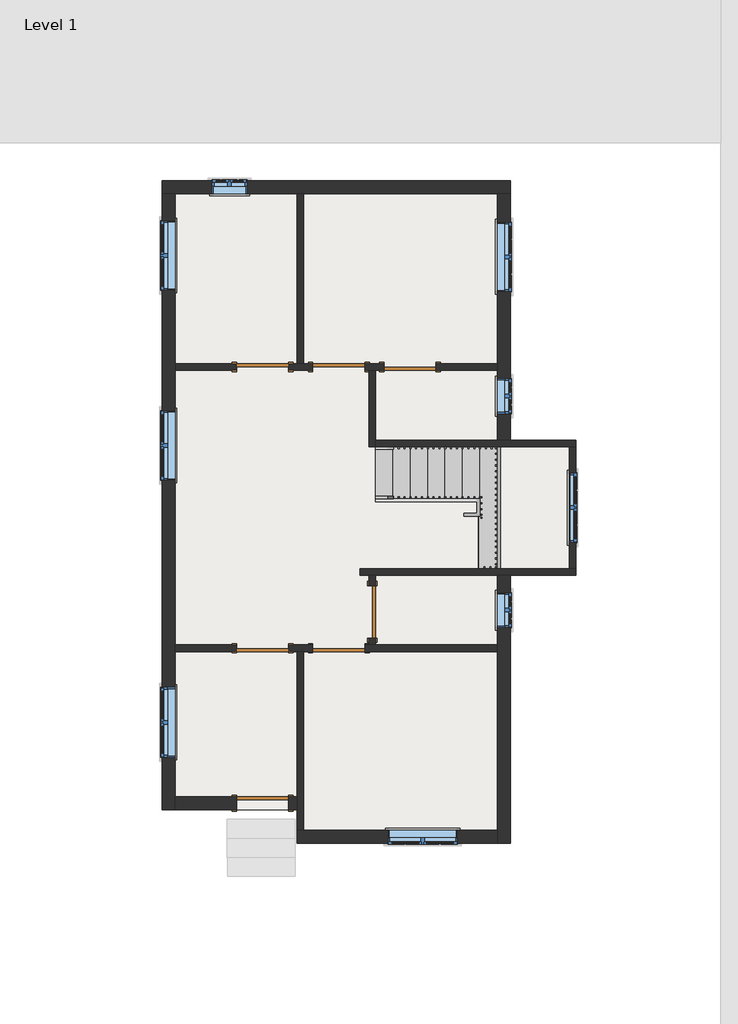
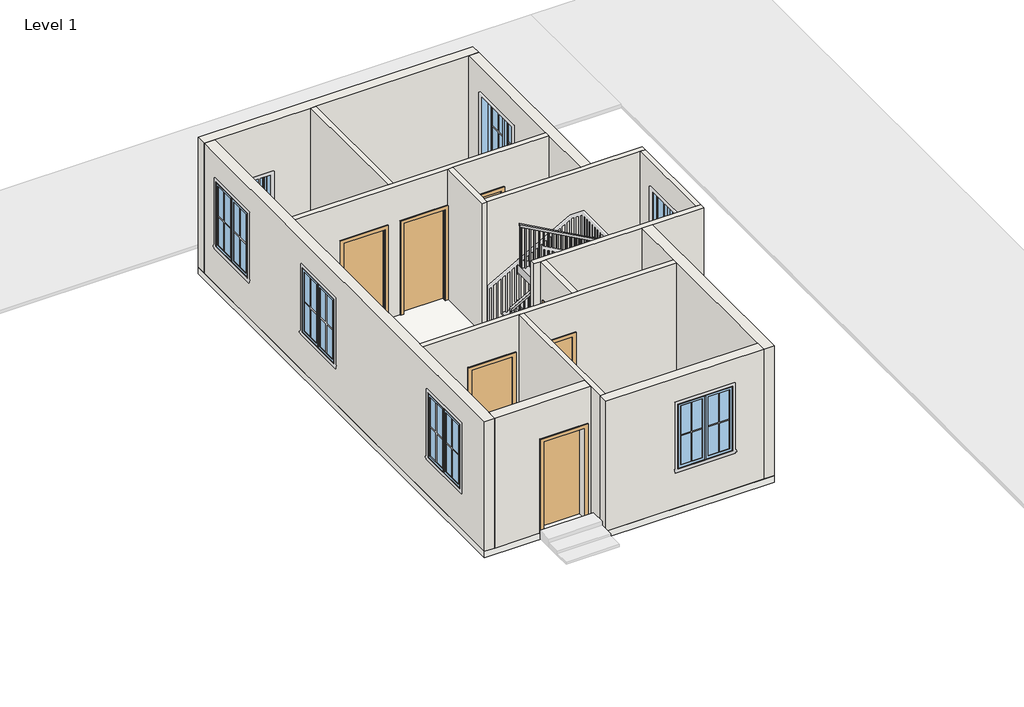
# One storey, part 1 of 2: 15 walls, 9 windows, 7 doors, 1 railing, 1 slab, 1 stair flight.
"""IFC4 building model written with IfcOpenShell, lengths in millimetres."""

from ifc_helpers import new_model, si_unit, frame, origin, origin_with_axes, place, context, project, spatial, polyline, outline, extrude, faceted_brep, transform, mapped, element, save
from components import door_e5f9f3c4, door_305aa2a5, door_0ca8825f, stair_flight_65dd4c8f, window_c417fced, window_8377141f, window_d9d3dda5

model = new_model("IFC4")

# Units and contexts
model_context = context("Model", 3, world=origin())
ifc_project = project(units=[si_unit("LENGTHUNIT", "METRE", prefix="MILLI")], contexts=[model_context])

# Site, building, storey
site = spatial("IfcSite", under=ifc_project)
building = spatial("IfcBuilding", under=site)
storey = spatial("IfcBuildingStorey", under=building, Name="Level 1", Elevation=0.0)

# Doors
placement = place(None, origin())
door_shape = door_e5f9f3c4(model_context)
element("IfcDoor", 1, ObjectType="Single-Flush : 36\" x 84\"", at=placement, inside=storey, context=model_context, shape_type="MappedRepresentation", body=[
    mapped(door_shape, transform((3028.95, 10966.45, 0.0), x_axis=(1.0, 0.0, 0.0), y_axis=(0.0, 1.0, 0.0), z_axis=(0.0, 0.0, 1.0))),
])
element("IfcDoor", 2, ObjectType="Single-Flush : 36\" x 84\"", at=placement, inside=storey, context=model_context, shape_type="MappedRepresentation", body=[
    mapped(door_shape, transform((5607.05, 10966.45, 0.0), x_axis=(-1.0, 0.0, 0.0), y_axis=(0.0, -1.0, 0.0), z_axis=(0.0, 0.0, 1.0))),
])
element("IfcDoor", 3, ObjectType="Single-Flush : 36\" x 84\"", at=placement, inside=storey, context=model_context, shape_type="MappedRepresentation", body=[
    mapped(door_shape, transform((4362.45, 6051.55, 0.0), x_axis=(-1.0, 0.0, 0.0), y_axis=(0.0, -1.0, 0.0), z_axis=(0.0, 0.0, 1.0))),
])
element("IfcDoor", 4, ObjectType="Single-Flush : 36\" x 84\"", at=placement, inside=storey, context=model_context, shape_type="MappedRepresentation", body=[
    mapped(door_shape, transform((4946.65, 6686.55, 0.0), x_axis=(0.0, -1.0, 0.0), y_axis=(1.0, 0.0, 0.0), z_axis=(0.0, 0.0, 1.0))),
])
door_2_shape = door_305aa2a5(model_context)
element("IfcDoor", 5, ObjectType="Single-Flush : 36\" x 84\"", at=placement, inside=storey, context=model_context, shape_type="MappedRepresentation", body=[
    mapped(door_2_shape, transform((4362.45, 10966.45, 0.0), x_axis=(-1.0, 0.0, 0.0), y_axis=(0.0, -1.0, 0.0), z_axis=(0.0, 0.0, 1.0))),
])
element("IfcDoor", 6, ObjectType="Single-Flush : 36\" x 84\"", at=placement, inside=storey, context=model_context, shape_type="MappedRepresentation", body=[
    mapped(door_2_shape, transform((3028.95, 6051.55, 0.0), x_axis=(1.0, 0.0, 0.0), y_axis=(0.0, 1.0, 0.0), z_axis=(0.0, 0.0, 1.0))),
])
door_3_shape = door_0ca8825f(model_context)
element("IfcDoor", 7, ObjectType="Single-Flush : 36\" x 84\"", at=placement, inside=storey, context=model_context, shape_type="MappedRepresentation", body=[
    mapped(door_3_shape, transform((3028.95, 3340.1, 0.0), x_axis=(1.0, 0.0, 0.0), y_axis=(0.0, 1.0, 0.0), z_axis=(0.0, 0.0, 1.0))),
])

# Railing
element("IfcRailing", 8, ObjectType="Handrail - Rectangular", at=placement, inside=storey, context=model_context, shape_type="SolidModel", body=[
    faceted_brep([(5003.8, 8712.2, 1083.7333333), (5003.8, 8712.2, 1025.620221), (5003.8, 8661.4, 1025.620221), (5003.8, 8661.4, 1083.7333333), (6756.4, 8712.2, 2057.4), (6807.2, 8712.2, 2027.5091099), (6807.2, 8661.4, 2027.5091099), (6756.4, 8661.4, 2057.4), (6756.4, 8712.2, 2099.7333333), (6807.2, 8712.2, 2048.9333333), (6807.2, 8661.4, 2048.9333333), (6756.4, 8661.4, 2099.7333333), (6883.4, 8712.2, 2099.7333333), (6883.4, 8712.2, 2048.9333333), (6832.6, 8661.4, 2048.9333333), (6832.6, 8661.4, 2099.7333333), (6883.4, 8585.2, 2099.7333333), (6883.4, 8585.2, 2048.9333333), (6832.6, 8585.2, 2048.9333333), (6832.6, 8585.2, 2099.7333333), (6883.4, 8432.8, 2099.7333333), (6883.4, 8382.0, 2048.9333333), (6832.6, 8382.0, 2048.9333333), (6832.6, 8432.8, 2099.7333333), (6883.4, 8432.8, 2311.4), (6883.4, 8382.0, 2260.6), (6832.6, 8382.0, 2260.6), (6832.6, 8432.8, 2311.4), (6883.4, 8305.8, 2311.4), (6883.4, 8305.8, 2260.6), (6832.6, 8356.6, 2260.6), (6832.6, 8356.6, 2311.4), (6756.4, 8305.8, 2311.4), (6743.2363978, 8305.8, 2260.6), (6743.2363978, 8356.6, 2260.6), (6756.4, 8356.6, 2311.4), (5003.8, 8305.8, 3285.0666667), (5003.8, 8356.6, 3285.0666667), (5003.8, 8356.6, 3226.9535543), (5003.8, 8305.8, 3226.9535543)], [[[0, 1, 2, 3]], [[1, 0, 4, 5]], [[2, 1, 5, 6]], [[3, 2, 6, 7]], [[0, 3, 7, 4]], [[5, 4, 8, 9]], [[6, 5, 9, 10]], [[7, 6, 10, 11]], [[4, 7, 11, 8]], [[9, 8, 12, 13]], [[10, 9, 13, 14]], [[11, 10, 14, 15]], [[8, 11, 15, 12]], [[13, 12, 16, 17]], [[14, 13, 17, 18]], [[15, 14, 18, 19]], [[12, 15, 19, 16]], [[17, 16, 20, 21]], [[18, 17, 21, 22]], [[19, 18, 22, 23]], [[16, 19, 23, 20]], [[21, 20, 24, 25]], [[22, 21, 25, 26]], [[23, 22, 26, 27]], [[20, 23, 27, 24]], [[25, 24, 28, 29]], [[26, 25, 29, 30]], [[27, 26, 30, 31]], [[24, 27, 31, 28]], [[29, 28, 32, 33]], [[30, 29, 33, 34]], [[31, 30, 34, 35]], [[28, 31, 35, 32]], [[36, 37, 38, 39]], [[33, 32, 36, 39]], [[34, 33, 39, 38]], [[35, 34, 38, 37]], [[32, 35, 37, 36]]]),
    extrude(outline(polyline([(3207.5507765, 5038.725), (3218.1341099, 5019.675), (2201.3333333, 5019.675), (2201.3333333, 5038.725), (3207.5507765, 5038.725)])), frame((0.0, 8321.675, 0.0), z_axis=(0.0, 1.0, 0.0), x_axis=(0.0, 0.0, 1.0)), (0.0, 0.0, 1.0), 19.05),
    extrude(outline(polyline([(3151.1063321, 5140.325), (3161.6896654, 5121.275), (2201.3333333, 5121.275), (2201.3333333, 5140.325), (3151.1063321, 5140.325)])), frame((0.0, 8321.675, 0.0), z_axis=(0.0, 1.0, 0.0), x_axis=(0.0, 0.0, 1.0)), (0.0, 0.0, 1.0), 19.05),
    extrude(outline(polyline([(3094.6618876, 5241.925), (3105.245221, 5222.875), (2201.3333333, 5222.875), (2201.3333333, 5241.925), (3094.6618876, 5241.925)])), frame((0.0, 8321.675, 0.0), z_axis=(0.0, 1.0, 0.0), x_axis=(0.0, 0.0, 1.0)), (0.0, 0.0, 1.0), 19.05),
    extrude(outline(polyline([(3038.2174432, 5343.525), (3048.8007765, 5324.475), (2032.0, 5324.475), (2032.0, 5343.525), (3038.2174432, 5343.525)])), frame((0.0, 8321.675, 0.0), z_axis=(0.0, 1.0, 0.0), x_axis=(0.0, 0.0, 1.0)), (0.0, 0.0, 1.0), 19.05),
    extrude(outline(polyline([(2981.7729988, 5445.125), (2992.3563321, 5426.075), (2032.0, 5426.075), (2032.0, 5445.125), (2981.7729988, 5445.125)])), frame((0.0, 8321.675, 0.0), z_axis=(0.0, 1.0, 0.0), x_axis=(0.0, 0.0, 1.0)), (0.0, 0.0, 1.0), 19.05),
    extrude(outline(polyline([(2925.3285543, 5546.725), (2935.9118876, 5527.675), (2032.0, 5527.675), (2032.0, 5546.725), (2925.3285543, 5546.725)])), frame((0.0, 8321.675, 0.0), z_axis=(0.0, 1.0, 0.0), x_axis=(0.0, 0.0, 1.0)), (0.0, 0.0, 1.0), 19.05),
    extrude(outline(polyline([(2868.8841099, 5648.325), (2879.4674432, 5629.275), (1862.6666667, 5629.275), (1862.6666667, 5648.325), (2868.8841099, 5648.325)])), frame((0.0, 8321.675, 0.0), z_axis=(0.0, 1.0, 0.0), x_axis=(0.0, 0.0, 1.0)), (0.0, 0.0, 1.0), 19.05),
    extrude(outline(polyline([(2812.4396654, 5749.925), (2823.0229988, 5730.875), (1862.6666667, 5730.875), (1862.6666667, 5749.925), (2812.4396654, 5749.925)])), frame((0.0, 8321.675, 0.0), z_axis=(0.0, 1.0, 0.0), x_axis=(0.0, 0.0, 1.0)), (0.0, 0.0, 1.0), 19.05),
    extrude(outline(polyline([(2755.995221, 5851.525), (2766.5785543, 5832.475), (1862.6666667, 5832.475), (1862.6666667, 5851.525), (2755.995221, 5851.525)])), frame((0.0, 8321.675, 0.0), z_axis=(0.0, 1.0, 0.0), x_axis=(0.0, 0.0, 1.0)), (0.0, 0.0, 1.0), 19.05),
    extrude(outline(polyline([(2699.5507765, 5953.125), (2710.1341099, 5934.075), (1693.3333333, 5934.075), (1693.3333333, 5953.125), (2699.5507765, 5953.125)])), frame((0.0, 8321.675, 0.0), z_axis=(0.0, 1.0, 0.0), x_axis=(0.0, 0.0, 1.0)), (0.0, 0.0, 1.0), 19.05),
    extrude(outline(polyline([(2643.1063321, 6054.725), (2653.6896654, 6035.675), (1693.3333333, 6035.675), (1693.3333333, 6054.725), (2643.1063321, 6054.725)])), frame((0.0, 8321.675, 0.0), z_axis=(0.0, 1.0, 0.0), x_axis=(0.0, 0.0, 1.0)), (0.0, 0.0, 1.0), 19.05),
    extrude(outline(polyline([(2586.6618876, 6156.325), (2597.245221, 6137.275), (1693.3333333, 6137.275), (1693.3333333, 6156.325), (2586.6618876, 6156.325)])), frame((0.0, 8321.675, 0.0), z_axis=(0.0, 1.0, 0.0), x_axis=(0.0, 0.0, 1.0)), (0.0, 0.0, 1.0), 19.05),
    extrude(outline(polyline([(2530.2174432, 6257.925), (2540.8007765, 6238.875), (1524.0, 6238.875), (1524.0, 6257.925), (2530.2174432, 6257.925)])), frame((0.0, 8321.675, 0.0), z_axis=(0.0, 1.0, 0.0), x_axis=(0.0, 0.0, 1.0)), (0.0, 0.0, 1.0), 19.05),
    extrude(outline(polyline([(2473.7729988, 6359.525), (2484.3563321, 6340.475), (1524.0, 6340.475), (1524.0, 6359.525), (2473.7729988, 6359.525)])), frame((0.0, 8321.675, 0.0), z_axis=(0.0, 1.0, 0.0), x_axis=(0.0, 0.0, 1.0)), (0.0, 0.0, 1.0), 19.05),
    extrude(outline(polyline([(2417.3285543, 6461.125), (2427.9118876, 6442.075), (1524.0, 6442.075), (1524.0, 6461.125), (2417.3285543, 6461.125)])), frame((0.0, 8321.675, 0.0), z_axis=(0.0, 1.0, 0.0), x_axis=(0.0, 0.0, 1.0)), (0.0, 0.0, 1.0), 19.05),
    extrude(outline(polyline([(2360.8841099, 6562.725), (2371.4674432, 6543.675), (1354.6666667, 6543.675), (1354.6666667, 6562.725), (2360.8841099, 6562.725)])), frame((0.0, 8321.675, 0.0), z_axis=(0.0, 1.0, 0.0), x_axis=(0.0, 0.0, 1.0)), (0.0, 0.0, 1.0), 19.05),
    extrude(outline(polyline([(2304.4396654, 6664.325), (2315.0229988, 6645.275), (1354.6666667, 6645.275), (1354.6666667, 6664.325), (2304.4396654, 6664.325)])), frame((0.0, 8321.675, 0.0), z_axis=(0.0, 1.0, 0.0), x_axis=(0.0, 0.0, 1.0)), (0.0, 0.0, 1.0), 19.05),
    extrude(outline(polyline([(2247.995221, 6765.925), (2258.5785543, 6746.875), (1354.6666667, 6746.875), (1354.6666667, 6765.925), (2247.995221, 6765.925)])), frame((0.0, 8321.675, 0.0), z_axis=(0.0, 1.0, 0.0), x_axis=(0.0, 0.0, 1.0)), (0.0, 0.0, 1.0), 19.05),
    extrude(outline(polyline([(6848.475, 8391.525), (6867.525, 8391.525), (6867.525, 8372.475), (6848.475, 8372.475), (6848.475, 8391.525)])), frame((0.0, 0.0, 1185.3333333), z_axis=(0.0, 0.0, 1.0), x_axis=(1.0, 0.0, 0.0)), (0.0, 0.0, 1.0), 1075.2666667),
    extrude(outline(polyline([(6848.475, 8493.125), (6867.525, 8493.125), (6867.525, 8474.075), (6848.475, 8474.075), (6848.475, 8493.125)])), frame((0.0, 0.0, 1185.3333333), z_axis=(0.0, 0.0, 1.0), x_axis=(1.0, 0.0, 0.0)), (0.0, 0.0, 1.0), 863.6),
    extrude(outline(polyline([(6848.475, 8594.725), (6867.525, 8594.725), (6867.525, 8575.675), (6848.475, 8575.675), (6848.475, 8594.725)])), frame((0.0, 0.0, 1185.3333333), z_axis=(0.0, 0.0, 1.0), x_axis=(1.0, 0.0, 0.0)), (0.0, 0.0, 1.0), 863.6),
    extrude(outline(polyline([(6823.075, 8677.275), (6823.075, 8696.325), (6842.125, 8696.325), (6842.125, 8677.275), (6823.075, 8677.275)])), frame((0.0, 0.0, 1185.3333333), z_axis=(0.0, 0.0, 1.0), x_axis=(1.0, 0.0, 0.0)), (0.0, 0.0, 1.0), 863.6),
    extrude(outline(polyline([(1990.4674432, 6740.525), (1979.8841099, 6721.475), (1016.0, 6721.475), (1016.0, 6740.525), (1990.4674432, 6740.525)])), frame((0.0, 8677.275, 0.0), z_axis=(0.0, 1.0, 0.0), x_axis=(0.0, 0.0, 1.0)), (0.0, 0.0, 1.0), 19.05),
    extrude(outline(polyline([(1934.0229988, 6638.925), (1923.4396654, 6619.875), (1016.0, 6619.875), (1016.0, 6638.925), (1934.0229988, 6638.925)])), frame((0.0, 8677.275, 0.0), z_axis=(0.0, 1.0, 0.0), x_axis=(0.0, 0.0, 1.0)), (0.0, 0.0, 1.0), 19.05),
    extrude(outline(polyline([(1877.5785543, 6537.325), (1866.995221, 6518.275), (1016.0, 6518.275), (1016.0, 6537.325), (1877.5785543, 6537.325)])), frame((0.0, 8677.275, 0.0), z_axis=(0.0, 1.0, 0.0), x_axis=(0.0, 0.0, 1.0)), (0.0, 0.0, 1.0), 19.05),
    extrude(outline(polyline([(1821.1341099, 6435.725), (1810.5507765, 6416.675), (846.6666667, 6416.675), (846.6666667, 6435.725), (1821.1341099, 6435.725)])), frame((0.0, 8677.275, 0.0), z_axis=(0.0, 1.0, 0.0), x_axis=(0.0, 0.0, 1.0)), (0.0, 0.0, 1.0), 19.05),
    extrude(outline(polyline([(1764.6896654, 6334.125), (1754.1063321, 6315.075), (846.6666667, 6315.075), (846.6666667, 6334.125), (1764.6896654, 6334.125)])), frame((0.0, 8677.275, 0.0), z_axis=(0.0, 1.0, 0.0), x_axis=(0.0, 0.0, 1.0)), (0.0, 0.0, 1.0), 19.05),
    extrude(outline(polyline([(1708.245221, 6232.525), (1697.6618876, 6213.475), (846.6666667, 6213.475), (846.6666667, 6232.525), (1708.245221, 6232.525)])), frame((0.0, 8677.275, 0.0), z_axis=(0.0, 1.0, 0.0), x_axis=(0.0, 0.0, 1.0)), (0.0, 0.0, 1.0), 19.05),
    extrude(outline(polyline([(1651.8007765, 6130.925), (1641.2174432, 6111.875), (677.3333333, 6111.875), (677.3333333, 6130.925), (1651.8007765, 6130.925)])), frame((0.0, 8677.275, 0.0), z_axis=(0.0, 1.0, 0.0), x_axis=(0.0, 0.0, 1.0)), (0.0, 0.0, 1.0), 19.05),
    extrude(outline(polyline([(1595.3563321, 6029.325), (1584.7729988, 6010.275), (677.3333333, 6010.275), (677.3333333, 6029.325), (1595.3563321, 6029.325)])), frame((0.0, 8677.275, 0.0), z_axis=(0.0, 1.0, 0.0), x_axis=(0.0, 0.0, 1.0)), (0.0, 0.0, 1.0), 19.05),
    extrude(outline(polyline([(1538.9118876, 5927.725), (1528.3285543, 5908.675), (677.3333333, 5908.675), (677.3333333, 5927.725), (1538.9118876, 5927.725)])), frame((0.0, 8677.275, 0.0), z_axis=(0.0, 1.0, 0.0), x_axis=(0.0, 0.0, 1.0)), (0.0, 0.0, 1.0), 19.05),
    extrude(outline(polyline([(1482.4674432, 5826.125), (1471.8841099, 5807.075), (508.0, 5807.075), (508.0, 5826.125), (1482.4674432, 5826.125)])), frame((0.0, 8677.275, 0.0), z_axis=(0.0, 1.0, 0.0), x_axis=(0.0, 0.0, 1.0)), (0.0, 0.0, 1.0), 19.05),
    extrude(outline(polyline([(1426.0229988, 5724.525), (1415.4396654, 5705.475), (508.0, 5705.475), (508.0, 5724.525), (1426.0229988, 5724.525)])), frame((0.0, 8677.275, 0.0), z_axis=(0.0, 1.0, 0.0), x_axis=(0.0, 0.0, 1.0)), (0.0, 0.0, 1.0), 19.05),
    extrude(outline(polyline([(1369.5785543, 5622.925), (1358.995221, 5603.875), (508.0, 5603.875), (508.0, 5622.925), (1369.5785543, 5622.925)])), frame((0.0, 8677.275, 0.0), z_axis=(0.0, 1.0, 0.0), x_axis=(0.0, 0.0, 1.0)), (0.0, 0.0, 1.0), 19.05),
    extrude(outline(polyline([(1313.1341099, 5521.325), (1302.5507765, 5502.275), (338.6666667, 5502.275), (338.6666667, 5521.325), (1313.1341099, 5521.325)])), frame((0.0, 8677.275, 0.0), z_axis=(0.0, 1.0, 0.0), x_axis=(0.0, 0.0, 1.0)), (0.0, 0.0, 1.0), 19.05),
    extrude(outline(polyline([(1256.6896654, 5419.725), (1246.1063321, 5400.675), (338.6666667, 5400.675), (338.6666667, 5419.725), (1256.6896654, 5419.725)])), frame((0.0, 8677.275, 0.0), z_axis=(0.0, 1.0, 0.0), x_axis=(0.0, 0.0, 1.0)), (0.0, 0.0, 1.0), 19.05),
    extrude(outline(polyline([(1200.245221, 5318.125), (1189.6618876, 5299.075), (338.6666667, 5299.075), (338.6666667, 5318.125), (1200.245221, 5318.125)])), frame((0.0, 8677.275, 0.0), z_axis=(0.0, 1.0, 0.0), x_axis=(0.0, 0.0, 1.0)), (0.0, 0.0, 1.0), 19.05),
    extrude(outline(polyline([(1143.8007765, 5216.525), (1133.2174432, 5197.475), (169.3333333, 5197.475), (169.3333333, 5216.525), (1143.8007765, 5216.525)])), frame((0.0, 8677.275, 0.0), z_axis=(0.0, 1.0, 0.0), x_axis=(0.0, 0.0, 1.0)), (0.0, 0.0, 1.0), 19.05),
    extrude(outline(polyline([(1087.3563321, 5114.925), (1076.7729988, 5095.875), (169.3333333, 5095.875), (169.3333333, 5114.925), (1087.3563321, 5114.925)])), frame((0.0, 8677.275, 0.0), z_axis=(0.0, 1.0, 0.0), x_axis=(0.0, 0.0, 1.0)), (0.0, 0.0, 1.0), 19.05),
    extrude(outline(polyline([(6848.475, 8340.725), (6867.525, 8340.725), (6867.525, 8321.675), (6848.475, 8321.675), (6848.475, 8340.725)])), frame((0.0, 0.0, 1185.3333333), z_axis=(0.0, 0.0, 1.0), x_axis=(1.0, 0.0, 0.0)), (0.0, 0.0, 1.0), 1075.2666667),
    extrude(outline(polyline([(6848.475, 8677.275), (6848.475, 8696.325), (6867.525, 8696.325), (6867.525, 8677.275), (6848.475, 8677.275)])), frame((0.0, 0.0, 1185.3333333), z_axis=(0.0, 0.0, 1.0), x_axis=(1.0, 0.0, 0.0)), (0.0, 0.0, 1.0), 863.6),
    extrude(outline(polyline([(3216.370221, 5022.85), (3226.9535543, 5003.8), (2201.3333333, 5003.8), (2201.3333333, 5022.85), (3216.370221, 5022.85)])), frame((0.0, 8321.675, 0.0), z_axis=(0.0, 1.0, 0.0), x_axis=(0.0, 0.0, 1.0)), (0.0, 0.0, 1.0), 19.05),
    extrude(outline(polyline([(1036.2035543, 5022.85), (1025.620221, 5003.8), (169.3333333, 5003.8), (169.3333333, 5022.85), (1036.2035543, 5022.85)])), frame((0.0, 8677.275, 0.0), z_axis=(0.0, 1.0, 0.0), x_axis=(0.0, 0.0, 1.0)), (0.0, 0.0, 1.0), 19.05),
])

# Slab
element("IfcSlab", 9, ObjectType="Generic - 12\"", at=placement, inside=storey, context=model_context, shape_type="SweptSolid", body=[
    extrude(outline(polyline([(7366.0, 14224.0), (7366.0, 9690.1), (8509.0, 9690.1), (8509.0, 7327.9), (7366.0, 7327.9), (7366.0, 2641.6), (3632.2, 2641.6), (3632.2, 3225.8), (1270.0, 3225.8), (1270.0, 14224.0), (7366.0, 14224.0)])), frame((0.0, 0.0, -152.4), z_axis=(0.0, 0.0, 1.0), x_axis=(1.0, 0.0, 0.0)), (0.0, 0.0, 1.0), 152.4),
])

# Stair flight
stair_flight_shape = stair_flight_65dd4c8f(model_context)
element("IfcStairFlight", 10, ObjectType="2\" Tread 1\" Nosing 1/4\" Riser", at=placement, inside=storey, context=model_context, shape_type="MappedRepresentation", body=[
    mapped(stair_flight_shape, transform((0.0, 0.0, 0.0), x_axis=(1.0, 0.0, 0.0), y_axis=(0.0, 1.0, 0.0), z_axis=(0.0, 0.0, 1.0))),
])

# Walls
element("IfcWall", 11, ObjectType="Generic - 5\"", at=placement, inside=storey, context=model_context, shape_type="Brep", body=[
    faceted_brep([(3486.15, 5994.4, 2133.6), (3486.15, 5994.4, 0.0), (3632.2, 5994.4, 0.0), (3746.5, 5994.4, 0.0), (3905.25, 5994.4, 0.0), (3905.25, 5994.4, 2133.6), (4819.65, 5994.4, 2133.6), (4819.65, 5994.4, 0.0), (7137.4, 5994.4, 0.0), (7137.4, 5994.4, 3048.0), (3746.5, 5994.4, 3048.0), (3632.2, 5994.4, 3048.0), (1498.6, 5994.4, 3048.0), (1498.6, 5994.4, 0.0), (2571.75, 5994.4, 0.0), (2571.75, 5994.4, 2133.6), (3905.25, 6108.7, 0.0), (3486.15, 6108.7, 0.0), (3486.15, 6108.7, 2133.6), (2571.75, 6108.7, 2133.6), (2571.75, 6108.7, 0.0), (1498.6, 6108.7, 0.0), (1498.6, 6108.7, 3048.0), (4889.5, 6108.7, 3048.0), (5003.8, 6108.7, 3048.0), (7137.4, 6108.7, 3048.0), (7137.4, 6108.7, 0.0), (5003.8, 6108.7, 0.0), (4889.5, 6108.7, 0.0), (4819.65, 6108.7, 0.0), (4819.65, 6108.7, 2133.6), (3905.25, 6108.7, 2133.6)], [[[0, 1, 2, 3, 4, 5, 6, 7, 8, 9, 10, 11, 12, 13, 14, 15]], [[16, 17, 18, 19, 20, 21, 22, 23, 24, 25, 26, 27, 28, 29, 30, 31]], [[29, 28, 27, 26, 8, 7]], [[14, 13, 21, 20]], [[4, 3, 2, 1, 17, 16]], [[12, 11, 10, 9, 25, 24, 23, 22]], [[13, 12, 22, 21]], [[9, 8, 26, 25]], [[5, 4, 16, 31]], [[6, 5, 31, 30]], [[7, 6, 30, 29]], [[18, 17, 1, 0]], [[19, 18, 0, 15]], [[20, 19, 15, 14]]]),
])
element("IfcWall", 12, ObjectType="Generic - 5\"", at=placement, inside=storey, context=model_context, shape_type="Brep", body=[
    faceted_brep([(3632.2, 5994.4, 0.0), (3632.2, 3454.4, 0.0), (3632.2, 3225.8, 0.0), (3632.2, 2870.2, 0.0), (3632.2, 2870.2, 3048.0), (3632.2, 3225.8, 3048.0), (3632.2, 3454.4, 3048.0), (3632.2, 5994.4, 3048.0), (3746.5, 5994.4, 0.0), (3746.5, 5994.4, 3048.0), (3746.5, 2870.2, 3048.0), (3746.5, 2870.2, 0.0)], [[[0, 1, 2, 3, 4, 5, 6, 7]], [[8, 9, 10, 11]], [[3, 2, 1, 0, 8, 11]], [[7, 6, 5, 4, 10, 9]], [[4, 3, 11, 10]], [[0, 7, 9, 8]]]),
])
element("IfcWall", 13, ObjectType="Generic - 5\"", at=placement, inside=storey, context=model_context, shape_type="SweptSolid", body=[
    extrude(outline(polyline([(6229.35, 2133.6), (6229.35, 0.0), (6108.7, 0.0), (6108.7, 3048.0), (7327.9, 3048.0), (7327.9, 0.0), (7143.75, 0.0), (7143.75, 2133.6), (6229.35, 2133.6)])), frame((4889.5, 0.0, 0.0), z_axis=(1.0, 0.0, 0.0), x_axis=(0.0, 1.0, 0.0)), (0.0, 0.0, 1.0), 114.3),
])
element("IfcWall", 14, ObjectType="Generic - 5\"", at=placement, inside=storey, context=model_context, shape_type="Brep", body=[
    faceted_brep([(4737.1, 7327.9, 0.0), (4889.5, 7327.9, 0.0), (5003.8, 7327.9, 0.0), (7137.4, 7327.9, 0.0), (7366.0, 7327.9, 0.0), (8509.0, 7327.9, 0.0), (8509.0, 7327.9, 3048.0), (7366.0, 7327.9, 3048.0), (7137.4, 7327.9, 3048.0), (5003.8, 7327.9, 3048.0), (4889.5, 7327.9, 3048.0), (4737.1, 7327.9, 3048.0), (4737.1, 7442.2, 0.0), (4737.1, 7442.2, 3048.0), (8394.7, 7442.2, 3048.0), (8509.0, 7442.2, 3048.0), (8509.0, 7442.2, 0.0), (8394.7, 7442.2, 0.0)], [[[0, 1, 2, 3, 4, 5, 6, 7, 8, 9, 10, 11]], [[12, 13, 14, 15, 16, 17]], [[5, 4, 3, 2, 1, 0, 12, 17, 16]], [[11, 10, 9, 8, 7, 6, 15, 14, 13]], [[0, 11, 13, 12]], [[6, 5, 16, 15]]]),
])
element("IfcWall", 15, ObjectType="Generic - 5\"", at=placement, inside=storey, context=model_context, shape_type="Brep", body=[
    faceted_brep([(4819.65, 10909.3, 0.0), (4889.5, 10909.3, 0.0), (5003.8, 10909.3, 0.0), (5149.85, 10909.3, 0.0), (5149.85, 10909.3, 2133.6), (6064.25, 10909.3, 2133.6), (6064.25, 10909.3, 0.0), (7137.4, 10909.3, 0.0), (7137.4, 10909.3, 3048.0), (5003.8, 10909.3, 3048.0), (4889.5, 10909.3, 3048.0), (1498.6, 10909.3, 3048.0), (1498.6, 10909.3, 0.0), (2571.75, 10909.3, 0.0), (2571.75, 10909.3, 2133.6), (3486.15, 10909.3, 2133.6), (3486.15, 10909.3, 0.0), (3905.25, 10909.3, 0.0), (3905.25, 10909.3, 2133.6), (4819.65, 10909.3, 2133.6), (5149.85, 11023.6, 2133.6), (5149.85, 11023.6, 0.0), (4819.65, 11023.6, 0.0), (4819.65, 11023.6, 2133.6), (3905.25, 11023.6, 2133.6), (3905.25, 11023.6, 0.0), (3746.5, 11023.6, 0.0), (3632.2, 11023.6, 0.0), (3486.15, 11023.6, 0.0), (3486.15, 11023.6, 2133.6), (2571.75, 11023.6, 2133.6), (2571.75, 11023.6, 0.0), (1498.6, 11023.6, 0.0), (1498.6, 11023.6, 3048.0), (3632.2, 11023.6, 3048.0), (3746.5, 11023.6, 3048.0), (7137.4, 11023.6, 3048.0), (7137.4, 11023.6, 0.0), (6064.25, 11023.6, 0.0), (6064.25, 11023.6, 2133.6)], [[[0, 1, 2, 3, 4, 5, 6, 7, 8, 9, 10, 11, 12, 13, 14, 15, 16, 17, 18, 19]], [[20, 21, 22, 23, 24, 25, 26, 27, 28, 29, 30, 31, 32, 33, 34, 35, 36, 37, 38, 39]], [[13, 12, 32, 31]], [[28, 27, 26, 25, 17, 16]], [[38, 37, 7, 6]], [[22, 21, 3, 2, 1, 0]], [[11, 10, 9, 8, 36, 35, 34, 33]], [[8, 7, 37, 36]], [[12, 11, 33, 32]], [[29, 28, 16, 15]], [[30, 29, 15, 14]], [[31, 30, 14, 13]], [[18, 17, 25, 24]], [[19, 18, 24, 23]], [[0, 19, 23, 22]], [[4, 3, 21, 20]], [[5, 4, 20, 39]], [[6, 5, 39, 38]]]),
])
element("IfcWall", 16, ObjectType="Generic - 5\"", at=placement, inside=storey, context=model_context, shape_type="Brep", body=[
    faceted_brep([(4889.5, 10909.3, 0.0), (4889.5, 9575.8, 0.0), (4889.5, 9575.8, 3048.0), (4889.5, 10909.3, 3048.0), (5003.8, 10909.3, 0.0), (5003.8, 10909.3, 3048.0), (5003.8, 9690.1, 3048.0), (5003.8, 9575.8, 3048.0), (5003.8, 9575.8, 0.0), (5003.8, 9690.1, 0.0)], [[[0, 1, 2, 3]], [[4, 5, 6, 7, 8, 9]], [[1, 0, 4, 9, 8]], [[3, 2, 7, 6, 5]], [[0, 3, 5, 4]], [[2, 1, 8, 7]]]),
])
element("IfcWall", 17, ObjectType="Generic - 5\"", at=placement, inside=storey, context=model_context, shape_type="Brep", body=[
    faceted_brep([(5003.8, 9575.8, 0.0), (8394.7, 9575.8, 0.0), (8509.0, 9575.8, 0.0), (8509.0, 9575.8, 3048.0), (8394.7, 9575.8, 3048.0), (5003.8, 9575.8, 3048.0), (5003.8, 9690.1, 0.0), (5003.8, 9690.1, 3048.0), (7137.4, 9690.1, 3048.0), (7366.0, 9690.1, 3048.0), (8509.0, 9690.1, 3048.0), (8509.0, 9690.1, 0.0), (7366.0, 9690.1, 0.0), (7137.4, 9690.1, 0.0)], [[[0, 1, 2, 3, 4, 5]], [[6, 7, 8, 9, 10, 11, 12, 13]], [[2, 1, 0, 6, 13, 12, 11]], [[5, 4, 3, 10, 9, 8, 7]], [[0, 5, 7, 6]], [[3, 2, 11, 10]]]),
])
element("IfcWall", 18, ObjectType="Generic - 5\"", at=placement, inside=storey, context=model_context, shape_type="SweptSolid", body=[
    extrude(outline(polyline([(9575.8, 0.0), (7442.2, 0.0), (7442.2, 3048.0), (9575.8, 3048.0), (9575.8, 0.0)]), holes=[polyline([(7899.4, 2438.4), (7899.4, 914.4), (9118.6, 914.4), (9118.6, 2438.4), (7899.4, 2438.4)])]), frame((8394.7, 0.0, 0.0), z_axis=(1.0, 0.0, 0.0), x_axis=(0.0, 1.0, 0.0)), (0.0, 0.0, 1.0), 114.3),
])
element("IfcWall", 19, ObjectType="Generic - 5\"", at=placement, inside=storey, context=model_context, shape_type="SweptSolid", body=[
    extrude(outline(polyline([(3632.2, 11023.6), (3632.2, 13995.4), (3746.5, 13995.4), (3746.5, 11023.6), (3632.2, 11023.6)])), origin_with_axes(), (0.0, 0.0, 1.0), 3048.0),
])
element("IfcWall", 20, ObjectType="Generic - 8\"", at=placement, inside=storey, context=model_context, shape_type="Brep", body=[
    faceted_brep([(1270.0, 13995.4, 0.0), (1498.6, 13995.4, 0.0), (3632.2, 13995.4, 0.0), (3746.5, 13995.4, 0.0), (7137.4, 13995.4, 0.0), (7366.0, 13995.4, 0.0), (7366.0, 13995.4, 3048.0), (7137.4, 13995.4, 3048.0), (3746.5, 13995.4, 3048.0), (3632.2, 13995.4, 3048.0), (1498.6, 13995.4, 3048.0), (1270.0, 13995.4, 3048.0), (2755.9, 13995.4, 1828.8), (2755.9, 13995.4, 914.4), (2146.3, 13995.4, 914.4), (2146.3, 13995.4, 1828.8), (1270.0, 14224.0, 0.0), (1270.0, 14224.0, 3048.0), (7366.0, 14224.0, 3048.0), (7366.0, 14224.0, 0.0), (2755.9, 14224.0, 1828.8), (2146.3, 14224.0, 1828.8), (2146.3, 14224.0, 914.4), (2755.9, 14224.0, 914.4)], [[[0, 1, 2, 3, 4, 5, 6, 7, 8, 9, 10, 11], [12, 13, 14, 15]], [[16, 17, 18, 19], [20, 21, 22, 23]], [[5, 4, 3, 2, 1, 0, 16, 19]], [[11, 10, 9, 8, 7, 6, 18, 17]], [[6, 5, 19, 18]], [[0, 11, 17, 16]], [[13, 12, 20, 23]], [[14, 13, 23, 22]], [[15, 14, 22, 21]], [[12, 15, 21, 20]]]),
])
element("IfcWall", 21, ObjectType="Generic - 8\"", at=placement, inside=storey, context=model_context, shape_type="Brep", body=[
    faceted_brep([(7137.4, 13995.4, 0.0), (7137.4, 11023.6, 0.0), (7137.4, 10909.3, 0.0), (7137.4, 9690.1, 0.0), (7137.4, 9690.1, 3048.0), (7137.4, 10909.3, 3048.0), (7137.4, 11023.6, 3048.0), (7137.4, 13995.4, 3048.0), (7137.4, 12280.9, 2438.4), (7137.4, 12280.9, 914.4), (7137.4, 13500.1, 914.4), (7137.4, 13500.1, 2438.4), (7137.4, 10153.65, 1828.8), (7137.4, 10153.65, 914.4), (7137.4, 10763.25, 914.4), (7137.4, 10763.25, 1828.8), (7366.0, 13995.4, 0.0), (7366.0, 13995.4, 3048.0), (7366.0, 9690.1, 3048.0), (7366.0, 9690.1, 0.0), (7366.0, 12280.9, 2438.4), (7366.0, 13500.1, 2438.4), (7366.0, 13500.1, 914.4), (7366.0, 12280.9, 914.4), (7366.0, 10153.65, 1828.8), (7366.0, 10763.25, 1828.8), (7366.0, 10763.25, 914.4), (7366.0, 10153.65, 914.4)], [[[0, 1, 2, 3, 4, 5, 6, 7], [8, 9, 10, 11], [12, 13, 14, 15]], [[16, 17, 18, 19], [20, 21, 22, 23], [24, 25, 26, 27]], [[3, 2, 1, 0, 16, 19]], [[7, 6, 5, 4, 18, 17]], [[0, 7, 17, 16]], [[4, 3, 19, 18]], [[9, 8, 20, 23]], [[10, 9, 23, 22]], [[11, 10, 22, 21]], [[8, 11, 21, 20]], [[13, 12, 24, 27]], [[14, 13, 27, 26]], [[15, 14, 26, 25]], [[12, 15, 25, 24]]]),
])
element("IfcWall", 22, ObjectType="Generic - 8\"", at=placement, inside=storey, context=model_context, shape_type="Brep", body=[
    faceted_brep([(1270.0, 13995.4, 0.0), (1270.0, 3225.8, 0.0), (1270.0, 3225.8, 3048.0), (1270.0, 13995.4, 3048.0), (1270.0, 13525.5, 2438.4), (1270.0, 12306.3, 2438.4), (1270.0, 12306.3, 914.4), (1270.0, 13525.5, 914.4), (1270.0, 5365.75, 2438.4), (1270.0, 4146.55, 2438.4), (1270.0, 4146.55, 914.4), (1270.0, 5365.75, 914.4), (1270.0, 10204.45, 2438.4), (1270.0, 8985.25, 2438.4), (1270.0, 8985.25, 914.4), (1270.0, 10204.45, 914.4), (1498.6, 13995.4, 0.0), (1498.6, 13995.4, 3048.0), (1498.6, 11023.6, 3048.0), (1498.6, 10909.3, 3048.0), (1498.6, 6108.7, 3048.0), (1498.6, 5994.4, 3048.0), (1498.6, 3454.4, 3048.0), (1498.6, 3225.8, 3048.0), (1498.6, 3225.8, 0.0), (1498.6, 3454.4, 0.0), (1498.6, 5994.4, 0.0), (1498.6, 6108.7, 0.0), (1498.6, 10909.3, 0.0), (1498.6, 11023.6, 0.0), (1498.6, 13525.5, 2438.4), (1498.6, 13525.5, 914.4), (1498.6, 12306.3, 914.4), (1498.6, 12306.3, 2438.4), (1498.6, 5365.75, 2438.4), (1498.6, 5365.75, 914.4), (1498.6, 4146.55, 914.4), (1498.6, 4146.55, 2438.4), (1498.6, 10204.45, 2438.4), (1498.6, 10204.45, 914.4), (1498.6, 8985.25, 914.4), (1498.6, 8985.25, 2438.4)], [[[0, 1, 2, 3], [4, 5, 6, 7], [8, 9, 10, 11], [12, 13, 14, 15]], [[16, 17, 18, 19, 20, 21, 22, 23, 24, 25, 26, 27, 28, 29], [30, 31, 32, 33], [34, 35, 36, 37], [38, 39, 40, 41]], [[1, 0, 16, 29, 28, 27, 26, 25, 24]], [[3, 2, 23, 22, 21, 20, 19, 18, 17]], [[0, 3, 17, 16]], [[2, 1, 24, 23]], [[31, 30, 4, 7]], [[32, 31, 7, 6]], [[33, 32, 6, 5]], [[30, 33, 5, 4]], [[35, 34, 8, 11]], [[36, 35, 11, 10]], [[37, 36, 10, 9]], [[34, 37, 9, 8]], [[39, 38, 12, 15]], [[40, 39, 15, 14]], [[41, 40, 14, 13]], [[38, 41, 13, 12]]]),
])
element("IfcWall", 23, ObjectType="Generic - 8\"", at=placement, inside=storey, context=model_context, shape_type="SweptSolid", body=[
    extrude(outline(polyline([(2133.6, 3486.15), (0.0, 3486.15), (0.0, 3632.2), (3048.0, 3632.2), (3048.0, 1498.6), (0.0, 1498.6), (0.0, 2571.75), (2133.6, 2571.75), (2133.6, 3486.15)])), frame((0.0, 3225.8, 0.0), z_axis=(0.0, 1.0, 0.0), x_axis=(0.0, 0.0, 1.0)), (0.0, 0.0, 1.0), 228.6),
])
element("IfcWall", 24, ObjectType="Generic - 8\"", at=placement, inside=storey, context=model_context, shape_type="Brep", body=[
    faceted_brep([(7137.4, 7327.9, 0.0), (7137.4, 6108.7, 0.0), (7137.4, 5994.4, 0.0), (7137.4, 2870.2, 0.0), (7137.4, 2641.6, 0.0), (7137.4, 2641.6, 3048.0), (7137.4, 2870.2, 3048.0), (7137.4, 5994.4, 3048.0), (7137.4, 6108.7, 3048.0), (7137.4, 7327.9, 3048.0), (7137.4, 6413.5, 1828.8), (7137.4, 6413.5, 914.4), (7137.4, 7023.1, 914.4), (7137.4, 7023.1, 1828.8), (7366.0, 7327.9, 0.0), (7366.0, 7327.9, 3048.0), (7366.0, 2641.6, 3048.0), (7366.0, 2641.6, 0.0), (7366.0, 6413.5, 1828.8), (7366.0, 7023.1, 1828.8), (7366.0, 7023.1, 914.4), (7366.0, 6413.5, 914.4)], [[[0, 1, 2, 3, 4, 5, 6, 7, 8, 9], [10, 11, 12, 13]], [[14, 15, 16, 17], [18, 19, 20, 21]], [[4, 3, 2, 1, 0, 14, 17]], [[9, 8, 7, 6, 5, 16, 15]], [[5, 4, 17, 16]], [[0, 9, 15, 14]], [[11, 10, 18, 21]], [[12, 11, 21, 20]], [[13, 12, 20, 19]], [[10, 13, 19, 18]]]),
])
element("IfcWall", 25, ObjectType="Generic - 8\"", at=placement, inside=storey, context=model_context, shape_type="Brep", body=[
    faceted_brep([(7137.4, 2870.2, 0.0), (3746.5, 2870.2, 0.0), (3632.2, 2870.2, 0.0), (3632.2, 2870.2, 3048.0), (3746.5, 2870.2, 3048.0), (7137.4, 2870.2, 3048.0), (5219.7, 2870.2, 2438.4), (5219.7, 2870.2, 914.4), (6438.9, 2870.2, 914.4), (6438.9, 2870.2, 2438.4), (7137.4, 2641.6, 0.0), (7137.4, 2641.6, 3048.0), (3632.2, 2641.6, 3048.0), (3632.2, 2641.6, 0.0), (5219.7, 2641.6, 2438.4), (6438.9, 2641.6, 2438.4), (6438.9, 2641.6, 914.4), (5219.7, 2641.6, 914.4)], [[[0, 1, 2, 3, 4, 5], [6, 7, 8, 9]], [[10, 11, 12, 13], [14, 15, 16, 17]], [[2, 1, 0, 10, 13]], [[5, 4, 3, 12, 11]], [[0, 5, 11, 10]], [[3, 2, 13, 12]], [[7, 6, 14, 17]], [[8, 7, 17, 16]], [[9, 8, 16, 15]], [[6, 9, 15, 14]]]),
])

# Windows
window_shape = window_c417fced(model_context)
element("IfcWindow", 26, ObjectType="Window-Casement-Double : 24\" x 36\"", at=placement, inside=storey, context=model_context, shape_type="MappedRepresentation", body=[
    mapped(window_shape, transform((2451.1, 14109.7, 0.0), x_axis=(1.0, 0.0, 0.0), y_axis=(0.0, 1.0, 0.0), z_axis=(0.0, 0.0, 1.0))),
])
element("IfcWindow", 27, ObjectType="Window-Casement-Double : 24\" x 36\"", at=placement, inside=storey, context=model_context, shape_type="MappedRepresentation", body=[
    mapped(window_shape, transform((7251.7, 10458.45, 0.0), x_axis=(0.0, -1.0, 0.0), y_axis=(1.0, 0.0, 0.0), z_axis=(0.0, 0.0, 1.0))),
])
element("IfcWindow", 28, ObjectType="Window-Casement-Double : 24\" x 36\"", at=placement, inside=storey, context=model_context, shape_type="MappedRepresentation", body=[
    mapped(window_shape, transform((7251.7, 6718.3, 0.0), x_axis=(0.0, -1.0, 0.0), y_axis=(1.0, 0.0, 0.0), z_axis=(0.0, 0.0, 1.0))),
])
window_2_shape = window_8377141f(model_context)
element("IfcWindow", 29, ObjectType="Window-Casement-Double : 48\" x 60\"", at=placement, inside=storey, context=model_context, shape_type="MappedRepresentation", body=[
    mapped(window_2_shape, transform((1384.3, 12915.9, 0.0), x_axis=(0.0, 1.0, 0.0), y_axis=(-1.0, 0.0, 0.0), z_axis=(0.0, 0.0, 1.0))),
])
element("IfcWindow", 30, ObjectType="Window-Casement-Double : 48\" x 60\"", at=placement, inside=storey, context=model_context, shape_type="MappedRepresentation", body=[
    mapped(window_2_shape, transform((7251.7, 12890.5, 0.0), x_axis=(0.0, -1.0, 0.0), y_axis=(1.0, 0.0, 0.0), z_axis=(0.0, 0.0, 1.0))),
])
element("IfcWindow", 31, ObjectType="Window-Casement-Double : 48\" x 60\"", at=placement, inside=storey, context=model_context, shape_type="MappedRepresentation", body=[
    mapped(window_2_shape, transform((5829.3, 2755.9, 0.0), x_axis=(-1.0, 0.0, 0.0), y_axis=(0.0, -1.0, 0.0), z_axis=(0.0, 0.0, 1.0))),
])
element("IfcWindow", 32, ObjectType="Window-Casement-Double : 48\" x 60\"", at=placement, inside=storey, context=model_context, shape_type="MappedRepresentation", body=[
    mapped(window_2_shape, transform((1384.3, 4756.15, 0.0), x_axis=(0.0, 1.0, 0.0), y_axis=(-1.0, 0.0, 0.0), z_axis=(0.0, 0.0, 1.0))),
])
element("IfcWindow", 33, ObjectType="Window-Casement-Double : 48\" x 60\"", at=placement, inside=storey, context=model_context, shape_type="MappedRepresentation", body=[
    mapped(window_2_shape, transform((1384.3, 9594.85, 0.0), x_axis=(0.0, 1.0, 0.0), y_axis=(-1.0, 0.0, 0.0), z_axis=(0.0, 0.0, 1.0))),
])
window_3_shape = window_d9d3dda5(model_context)
element("IfcWindow", 34, ObjectType="Window-Casement-Double : 48\" x 60\"", at=placement, inside=storey, context=model_context, shape_type="MappedRepresentation", body=[
    mapped(window_3_shape, transform((8451.85, 8509.0, 0.0), x_axis=(0.0, -1.0, 0.0), y_axis=(1.0, 0.0, 0.0), z_axis=(0.0, 0.0, 1.0))),
])

save(model, "model.ifc")

# Revit data of these elements
# Type "Single-Flush : 36\" x 84\""
#   Type Mark = "1"
#   Construction Type Id = "MDOOR"
#   Assembly Code = "C1020"
#   Analytic Construction = "Metal"
#   Thickness = 0' - 2"
#   Heat Transfer Coefficient (U) = 0.651978 BTU/(h·ft²·°F)
#   Height = 7' - 0"
#   Trim Projection Ext = 0' - 1"
#   Trim Projection Int = 0' - 1"
#   Trim Width = 0' - 3"
#   Width = 3' - 0"
#   Define Thermal Properties by = 1
#   Define Thermal Properties by = 1
#   Door Material = Door - Panel
#   Frame Material = Door - Frame
#   Visual Light Transmittance = 0
#   Solar Heat Gain Coefficient = 0
#   Function = (empty or 0)
#   Wall Closure = (empty or 0)
# Type "Handrail - Rectangular"
#   Assembly Code = "C2010400"
#   built-in parameter 1008612 = 0.0416667 (stored number, unit not read)
#   built-in parameter 1008611 = 0.0416667 (stored number, unit not read)
#   built-in parameter 1008609 = 0.333333 (stored number, unit not read)
#   built-in parameter 1008604 = 0.166667 (stored number, unit not read)
#   built-in parameter 1008603 = 0.166667 (stored number, unit not read)
#   Railing Height = 3' - 0"
#   built-in parameter 1008630 = 2
#   built-in parameter 1008610 = 2
#   built-in parameter 1008618 = Baluster - Square : 3/4"
# Type "Generic - 12\""
#   Assembly Code = "B1010"
#   Function = 0
#   Layers, outside or top first: 0' - 6" no material (function 1)
# Type "Generic - 5\""
#   Assembly Code = "B2010"
#   Layers, outside or top first: 0' - 4 1/2" no material (function 1)
# Type "Generic - 8\""
#   Assembly Code = "B2010"
#   Layers, outside or top first: 0' - 9" no material (function 1)
# Type "Window-Casement-Double : 24\" x 36\""
#   Type Mark = "14"
#   Fire Rating = "0.5h"
#   Assembly Code = "B2020100"
#   Analytic Construction = "Double glazing - domestic"
#   Frame Extension [instance default] = 0' - 0 1/4"
#   Window Inset [instance default] = 0' - 0"
#   Wall Thickness [instance default] = 0' - 6"
#   Interior Wall Closure [instance default] = 0' - 2 1/4"
#   Half Width = 1' - 0"
#   Visual Light Transmittance = 0.81
#   Thermal Resistance (R) = 1.8146 (h·ft²·°F)/BTU
#   Solar Heat Gain Coefficient = 0.76
#   Rough Width = 2' - 0 1/2"
#   Rough Height = 3' - 0 1/2"
#   Height = 3' - 0"
#   Heat Transfer Coefficient (U) = 0.5511 BTU/(h·ft²·°F)
#   Exterior Wall Closure [instance default] = 0' - 1 1/4"
#   Extension Jamb [instance default] = 0' - 2 1/4"
#   Default Sill Height = 3' - 0"
#   Width = 2' - 0"
#   Define Thermal Properties by = 0
#   Muntin Visibility = yes
#   Interior Trim Visibility [instance default] = yes
#   Exterior Trim Visibility [instance default] = yes
#   Extension Jamb Visibility [instance default] = yes
#   Interior Trim Material = Wood - Stained
#   Muntin Pattern = Muntin Pattern_2x2 : Muntin Pattern_2x2
#   Interior Trim = Trim-Window-Interior-Flat : Picture Frame
#   Interior Frame Material = Wood - Stained
#   Glass Panel Material = Glass
#   Exterior Trim Material = Clad - White
#   Exterior Trim = Trim-Window-Exterior-Flat : with Sill
#   Exterior Frame Material = Clad - White
#   Wall Closure = (empty or 0)
# Type "Window-Casement-Double : 48\" x 60\""
#   Type Mark = "17"
#   Fire Rating = "0.5h"
#   Assembly Code = "B2020100"
#   Analytic Construction = "Double glazing - domestic"
#   Frame Extension [instance default] = 0' - 0 1/4"
#   Window Inset [instance default] = 0' - 0"
#   Wall Thickness [instance default] = 0' - 6"
#   Interior Wall Closure [instance default] = 0' - 2 1/4"
#   Half Width = 2' - 0"
#   Visual Light Transmittance = 0.81
#   Thermal Resistance (R) = 1.8146 (h·ft²·°F)/BTU
#   Solar Heat Gain Coefficient = 0.76
#   Rough Width = 4' - 0 1/2"
#   Rough Height = 5' - 0 1/2"
#   Height = 5' - 0"
#   Heat Transfer Coefficient (U) = 0.5511 BTU/(h·ft²·°F)
#   Exterior Wall Closure [instance default] = 0' - 1 1/4"
#   Extension Jamb [instance default] = 0' - 2 1/4"
#   Default Sill Height = 3' - 0"
#   Width = 4' - 0"
#   Define Thermal Properties by = 0
#   Muntin Visibility = yes
#   Interior Trim Visibility [instance default] = yes
#   Exterior Trim Visibility [instance default] = yes
#   Extension Jamb Visibility [instance default] = yes
#   Interior Trim Material = Wood - Stained
#   Muntin Pattern = Muntin Pattern_2x2 : Muntin Pattern_2x2
#   Interior Trim = Trim-Window-Interior-Flat : Picture Frame
#   Interior Frame Material = Wood - Stained
#   Glass Panel Material = Glass
#   Exterior Trim Material = Clad - White
#   Exterior Trim = Trim-Window-Exterior-Flat : with Sill
#   Exterior Frame Material = Clad - White
#   Wall Closure = (empty or 0)
# Elements 1, 2, 3, 4, 5, 6, 7 (IfcDoor, "Single-Flush : 36\" x 84\"")
#   Phase Created = New Construction
#   Materials on its faces: "Door - Frame", "Door - Panel"
# Element 8 (IfcRailing, "Handrail - Rectangular")
#   Phase Created = New Construction
# Element 9 (IfcSlab, "Generic - 12\"")
#   Height Offset From Level = 0' - 0"
#   Phase Created = New Construction
#   Materials on its faces: "Clad - White", "Default Floor"
# Element 10 (IfcStairFlight, "2\" Tread 1\" Nosing 1/4\" Riser")
#   Phase Created = New Construction
# Elements 11, 13, 15, 16, 19 (IfcWall, "Generic - 5\"")
#   Top Offset = 0' - 0"
#   Base Offset = 0' - 0"
#   wall height = 10' - 0"
#   Phase Created = New Construction
#   Base Constraint = Level 1
#   Top Constraint = LEVEL2
#   Materials on its faces: "Default Wall"
# Elements 12, 14, 17, 18 (IfcWall, "Generic - 5\"")
#   Top Offset = 0' - 0"
#   Base Offset = 0' - 0"
#   wall height = 10' - 0"
#   Phase Created = New Construction
#   Base Constraint = Level 1
#   Top Constraint = LEVEL2
#   Materials on its faces: "Default Wall", "Parking Stripe"
# Elements 20, 21, 22, 24, 25 (IfcWall, "Generic - 8\"")
#   Top Offset = 0' - 0"
#   Base Offset = 0' - 0"
#   Unconnected Height = 10' - 0"
#   wall height = 10' - 0"
#   Phase Created = New Construction
#   Base Constraint = Level 1
#   Materials on its faces: "Default Wall", "Parking Stripe"
# Element 23 (IfcWall, "Generic - 8\"")
#   Top Offset = 0' - 0"
#   Base Offset = 0' - 0"
#   Unconnected Height = 10' - 0"
#   wall height = 10' - 0"
#   Phase Created = New Construction
#   Base Constraint = Level 1
#   Materials on its faces: "Default Wall", "Parking Stripe", "Door - Frame"
# Element 26 (IfcWindow, "Window-Casement-Double : 24\" x 36\"")
#   Mark = "7"
#   Window Inset = 0' - 0"
#   Interior Wall Closure = 0' - 2 1/4"
#   Frame Extension = 0' - 0 1/4"
#   Exterior Wall Closure = 0' - 1 1/4"
#   Interior Trim Visibility = yes
#   Exterior Trim Visibility = yes
#   Phase Created = New Construction
#   Materials on its faces: "Wood - Stained", "Glass", "Clad - White"
# Element 27 (IfcWindow, "Window-Casement-Double : 24\" x 36\"")
#   Mark = "8"
#   Window Inset = 0' - 0"
#   Interior Wall Closure = 0' - 2 1/4"
#   Frame Extension = 0' - 0 1/4"
#   Exterior Wall Closure = 0' - 1 1/4"
#   Interior Trim Visibility = yes
#   Exterior Trim Visibility = yes
#   Phase Created = New Construction
#   Materials on its faces: "Wood - Stained", "Glass", "Clad - White"
# Element 28 (IfcWindow, "Window-Casement-Double : 24\" x 36\"")
#   Mark = "9"
#   Window Inset = 0' - 0"
#   Interior Wall Closure = 0' - 2 1/4"
#   Frame Extension = 0' - 0 1/4"
#   Exterior Wall Closure = 0' - 1 1/4"
#   Interior Trim Visibility = yes
#   Exterior Trim Visibility = yes
#   Phase Created = New Construction
#   Materials on its faces: "Wood - Stained", "Glass", "Clad - White"
# Element 29 (IfcWindow, "Window-Casement-Double : 48\" x 60\"")
#   Mark = "1"
#   Window Inset = 0' - 0"
#   Interior Wall Closure = 0' - 2 1/4"
#   Frame Extension = 0' - 0 1/4"
#   Exterior Wall Closure = 0' - 1 1/4"
#   Interior Trim Visibility = yes
#   Exterior Trim Visibility = yes
#   Phase Created = New Construction
#   Materials on its faces: "Wood - Stained", "Glass", "Clad - White"
# Element 30 (IfcWindow, "Window-Casement-Double : 48\" x 60\"")
#   Mark = "2"
#   Window Inset = 0' - 0"
#   Interior Wall Closure = 0' - 2 1/4"
#   Frame Extension = 0' - 0 1/4"
#   Exterior Wall Closure = 0' - 1 1/4"
#   Interior Trim Visibility = yes
#   Exterior Trim Visibility = yes
#   Phase Created = New Construction
#   Materials on its faces: "Wood - Stained", "Glass", "Clad - White"
# Element 31 (IfcWindow, "Window-Casement-Double : 48\" x 60\"")
#   Mark = "4"
#   Window Inset = 0' - 0"
#   Interior Wall Closure = 0' - 2 1/4"
#   Frame Extension = 0' - 0 1/4"
#   Exterior Wall Closure = 0' - 1 1/4"
#   Interior Trim Visibility = yes
#   Exterior Trim Visibility = yes
#   Phase Created = New Construction
#   Materials on its faces: "Wood - Stained", "Glass", "Clad - White"
# Element 32 (IfcWindow, "Window-Casement-Double : 48\" x 60\"")
#   Mark = "5"
#   Window Inset = 0' - 0"
#   Interior Wall Closure = 0' - 2 1/4"
#   Frame Extension = 0' - 0 1/4"
#   Exterior Wall Closure = 0' - 1 1/4"
#   Interior Trim Visibility = yes
#   Exterior Trim Visibility = yes
#   Phase Created = New Construction
#   Materials on its faces: "Wood - Stained", "Glass", "Clad - White"
# Element 33 (IfcWindow, "Window-Casement-Double : 48\" x 60\"")
#   Mark = "6"
#   Window Inset = 0' - 0"
#   Interior Wall Closure = 0' - 2 1/4"
#   Frame Extension = 0' - 0 1/4"
#   Exterior Wall Closure = 0' - 1 1/4"
#   Interior Trim Visibility = yes
#   Exterior Trim Visibility = yes
#   Phase Created = New Construction
#   Materials on its faces: "Wood - Stained", "Glass", "Clad - White"
# Element 34 (IfcWindow, "Window-Casement-Double : 48\" x 60\"")
#   Mark = "3"
#   Window Inset = 0' - 0"
#   Interior Wall Closure = 0' - 2 1/4"
#   Frame Extension = 0' - 0 1/4"
#   Exterior Wall Closure = 0' - 1 1/4"
#   Interior Trim Visibility = yes
#   Exterior Trim Visibility = yes
#   Phase Created = New Construction
#   Materials on its faces: "Wood - Stained", "Glass", "Clad - White"
# Materials
#   "Door - Panel": class "Wood", colour RGB 210 159 95, transparency 0, Cost = 0
#   "Door - Frame": colour RGB 118 70 51, transparency 0, Cost = 0
#   "Wood - Stained": class "Wood", colour RGB 224 178 126, transparency 0, Cost = 0
#   "Glass": class "Glass", colour RGB 0 128 192, transparency 0.75, Description = "Soda Lime Glass", Cost = 0
#   "Clad - White": class "Wood", colour RGB 242 242 238, transparency 0, Cost = 0
#   "Default Floor": colour RGB 128 128 128, transparency 0, Cost = 0
#   "Default Wall": colour RGB 128 128 128, transparency 0, Cost = 0
#   "Parking Stripe": class "Paint", colour RGB 250 250 91, transparency 0, Cost = 0
